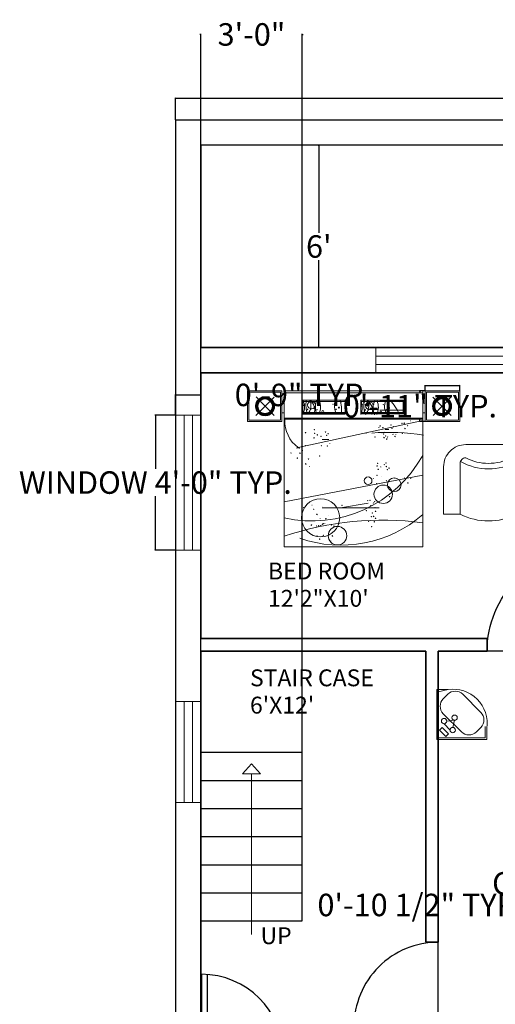
# Model space of a CAD drawing. Units: inches. Extents: x -11 to 443, y 65 to 743.
# Tile 7 of 10: x -11 to 158, y 392 to 743. Entities that reach past the tile are written whole.
import ezdxf

# ---------------------------------------------------------------- set-up
doc = ezdxf.new("R2010")
doc.units = ezdxf.units.IN
doc.header["$MEASUREMENT"] = 0
for name, color, linetype, lineweight in [('A-ANNO-DIMS', 2, 'Continuous', 18), ('A-ANNO-SYMB', 2, 'Continuous', 18), ('A-ANNO-TEXT', 2, 'Continuous', 18), ('A-AREA-IDEN', 2, 'Continuous', 18), ('A-DOOR', 4, 'Continuous', 25), ('A-FLOR-FIXT', 8, 'Continuous', 18), ('A-FLOR-STRS', 7, 'Continuous', 25), ('A-FURN-PATT', 8, 'Continuous', 9), ('A-GLAZ', 4, 'Continuous', 18), ('A-WALL', 7, 'Continuous', 35), ('A-WALL-SITE', 7, 'Continuous', 30), ('C-PROP', 3, 'Continuous', 30), ('Furniture', 7, 'Continuous', 15)]:
    doc.layers.add(name, color=color, linetype=linetype, lineweight=lineweight)
doc.styles.get("Standard").update_dxf_attribs({"font": 'italic8.shx'})
doc.dimstyles.get("Standard").update_dxf_attribs({"dimtxt": 8, "dimasz": 0.18, "dimexe": 0.18, "dimexo": 0.0625, "dimgap": 0.09, "dimtad": 0, "dimtih": 1, "dimtoh": 1, "dimzin": 0, "dimdsep": 46, "dimlunit": 3, "dimtxsty": 'Standard', "dimblk": 'CLOSEDBLANK', "dimcen": 0.09, "dimclrd": 6, "dimclre": 5, "dimclrt": 4, "dimadec": 0, "dimazin": 0, "dimtfac": 1, "dimtofl": 0, "dimtmove": 0, "dimatfit": 3, "dimfxl": 1, "dimtolj": 1, "dimtzin": 0, "dimarcsym": 0})

# ---------------------------------------------------------------- blocks, each defined once
blk = doc.blocks.new('_ClosedBlank')
at = {"color": 0, "linetype": 'ByBlock', "lineweight": -2}
for p, q in [((-1, 0.17), (0, 0)), ((-1, 0.17), (-1, -0.17)), ((0, 0), (-1, -0.17))]:
    blk.add_line(p, q, dxfattribs=at)
blk = doc.blocks.new('*D3')
at = {"layer": 'A-ANNO-DIMS', "color": 0, "lineweight": -2, "transparency": 16777216}
for p, q in [((95.1, 697.92), (94.99, 697.92)), ((95.17, 697.74), (95.17, 666.77)), ((95.17, 626.1), (95.17, 657.07)), ((95.1, 625.92), (94.99, 625.92))]:
    blk.add_line(p, q, dxfattribs=at)
at = {"layer": 'Defpoints', "color": 0, "lineweight": 100, "transparency": 16777216}
for p in [(95.17, 697.92), (95.17, 697.92), (95.17, 625.92)]:
    blk.add_point(p, dxfattribs=at)
at = {"layer": 'A-ANNO-DIMS', "color": 0, "lineweight": -2, "transparency": 16777216, "xscale": 0.18, "yscale": 0.18, "zscale": 0.18}
for p, rotation in [((95.17, 697.92), 90), ((95.17, 625.92), 270)]:
    blk.add_blockref('_ClosedBlank', p, dxfattribs=dict(at, rotation=rotation))
at = {"layer": 'A-ANNO-DIMS', "color": 0, "transparency": 16777216, "insert": (95.17, 661.92), "char_height": 8, "attachment_point": 5}
blk.add_mtext("\\A1;6'", dxfattribs=at)
blk = doc.blocks.new('*D5')
at = {"layer": 'A-ANNO-DIMS', "color": 0, "lineweight": -2, "transparency": 16777216}
for p, q in [((44.21, 706.98), (44.21, 714.84)), ((332.21, 706.98), (332.21, 714.84)), ((44.39, 714.66), (178.6, 714.66)), ((332.03, 714.66), (197.82, 714.66))]:
    blk.add_line(p, q, dxfattribs=at)
at = {"layer": 'Defpoints', "color": 0, "lineweight": 100, "transparency": 16777216}
for p in [(332.21, 714.66), (44.21, 706.92), (332.21, 706.92)]:
    blk.add_point(p, dxfattribs=at)
at = {"layer": 'A-ANNO-DIMS', "color": 0, "lineweight": -2, "transparency": 16777216, "xscale": 0.18, "yscale": 0.18, "zscale": 0.18, "rotation": 180}
blk.add_blockref('_ClosedBlank', (44.21, 714.66), dxfattribs=at)
at = {"layer": 'A-ANNO-DIMS', "color": 0, "lineweight": -2, "transparency": 16777216, "xscale": 0.18, "yscale": 0.18, "zscale": 0.18}
blk.add_blockref('_ClosedBlank', (332.21, 714.66), dxfattribs=at)
at = {"layer": 'A-ANNO-DIMS', "color": 0, "transparency": 16777216, "insert": (188.21, 714.66), "char_height": 8, "attachment_point": 5}
blk.add_mtext("\\A1;24'", dxfattribs=at)
blk = doc.blocks.new('DOOR-SWING-30')
for p, q in [((0, 30), (0, 0)), ((2, 29.93), (2, 0)), ((0, 0), (30, 0))]:
    blk.add_line(p, q)
blk.add_arc((0, 0), 30, 0, 90)
blk = doc.blocks.new('DOOR-SWING-36')
for p, q in [((36, 36), (0, 36)), ((0, 36), (0, 0)), ((35.94, 34), (0, 34))]:
    blk.add_line(p, q)
blk.add_arc((0, 36), 36, 270, 0)
blk = doc.blocks.new('WIN-48x9')
for p, q in [((0, 48), (0, 0)), ((9, 48), (0, 48)), ((3, 0), (3, 48)), ((6, 0), (6, 48)), ((9, 0), (9, 48)), ((0, 0), (9, 0))]:
    blk.add_line(p, q)
blk = doc.blocks.new('BED-DOUBLE')
for p, q in [((0.82, 54.51), (0, 54.51)), ((50.12, 55.53), (0.82, 55.53)), ((0.82, 55.53), (0.82, 0)), ((50.12, 54.78), (0.82, 54.78)), ((50.12, 0), (50.12, 55.53)), ((50.12, 0), (50.12, 55.53)), ((50.95, 54.51), (50.12, 54.51)), ((0.82, 51.08), (0, 51.08)), ((7.45, 52.2), (7.45, 47.27)), ((22.51, 52.2), (7.45, 52.2)), ((7.45, 51.71), (22.51, 51.71)), ((22.51, 47.27), (22.51, 52.2)), ((43.08, 52.21), (28.01, 52.21)), ((28.01, 52.21), (28.01, 47.28)), ((28.01, 51.71), (43.1, 51.71)), ((43.08, 52.14), (34.85, 52.14)), ((43.08, 47.28), (43.08, 52.21)), ((50.95, 51.08), (50.12, 51.08)), ((0.82, 47.66), (0, 47.66)), ((0.81, 45.69), (50.11, 45.69)), ((0.82, 45.79), (49.9, 45.79)), ((7.45, 47.77), (22.51, 47.77)), ((7.45, 47.56), (22.51, 47.56)), ((7.45, 47.35), (22.51, 47.35)), ((7.45, 47.27), (22.51, 47.27)), ((28.01, 47.77), (43.1, 47.77)), ((28.01, 47.56), (43.1, 47.56)), ((28.01, 47.35), (43.1, 47.35)), ((28.01, 47.28), (43.08, 47.28)), ((43.08, 48.66), (34.85, 48.66)), ((50.95, 47.66), (50.12, 47.66)), ((0.81, 45.48), (50.11, 45.48)), ((5.76, 35.31), (50.13, 44.94)), ((38, 41.71), (36.72, 41.71)), ((16.71, 38.23), (14.33, 38.23)), ((0.81, 16.07), (50.11, 25.52)), ((30.69, 15.53), (20.82, 13.88)), ((34.54, 13.88), (14.33, 13.88)), ((0.82, 0), (50.12, 0)), ((0.82, 0), (50.12, 0))]:
    blk.add_line(p, q)
for centre, radius in [((7.67, 50.33), 0.0548), ((7.99, 50.77), 0.0548), ((9.09, 50.77), 0.0548), ((10.51, 50.44), 1.37), ((10.62, 51.21), 0.0274), ((10.95, 51.64), 0.0274), ((12.05, 51.64), 0.0274), ((12.05, 50.88), 0.0274), ((18.18, 50.77), 0.0548), ((20.26, 49.56), 0.164), ((21.14, 51.64), 0.0274), ((28.25, 50.16), 0.0548), ((28.58, 50.6), 0.0548), ((29.68, 50.6), 0.0548), ((31.1, 50.27), 1.37), ((31.21, 51.03), 0.0274), ((31.53, 51.47), 0.0274), ((32.63, 51.47), 0.0274), ((32.63, 50.71), 0.0274), ((36.03, 50.6), 0.0548), ((38.11, 49.39), 0.164), ((41.72, 51.47), 0.0274), ((8.76, 48.47), 0.0822), ((9.09, 48.91), 0.0822), ((10.19, 48.91), 0.0822), ((12.48, 48.8), 0.0274), ((14.56, 48.14), 0.329), ((19.27, 48.91), 0.0822), ((29.35, 48.3), 0.0822), ((29.67, 48.74), 0.0822), ((30.77, 48.74), 0.0822), ((33.07, 48.63), 0.0274), ((35.15, 47.97), 0.329), ((37.12, 48.74), 0.0822), ((41.53, 45.6), 0.0822), ((34.49, 42.48), 0.0548), ((34.94, 42.97), 0.0822), ((35.9, 42.4), 0.0822), ((38.78, 43.35), 0.0822), ((39.16, 42.2), 0.0822), ((39.74, 42.78), 0.0822), ((42.72, 43.97), 0.0548), ((43.5, 44.01), 0.0822), ((43.81, 42.11), 0.0822), ((44.72, 43.1), 0.0274), ((45.68, 44.84), 0.0274), ((8.39, 40.62), 0.0822), ((11.37, 38.79), 0.0822), ((11.51, 41.72), 0.0548), ((11.65, 40.43), 0.0822), ((12.61, 39.86), 0.0822), ((13.92, 39.31), 0.0548), ((15.49, 40.82), 0.0822), ((15.87, 39.67), 0.0822), ((16.44, 40.24), 0.0822), ((29.94, 40.51), 0.0822), ((33.1, 39.09), 0.0822), ((35.59, 40.62), 0.0822), ((36.22, 40.19), 0.0548), ((36.35, 38.9), 0.0822), ((36.59, 41.14), 0.0274), ((36.93, 39.48), 0.0822), ((37.56, 39.06), 0.0548), ((39.48, 40), 0.0548), ((40.19, 39.28), 0.0822), ((40.52, 39.93), 0.0274), ((42.86, 40.37), 0.0822), ((5.33, 35.19), 0.0548), ((6.11, 35.23), 0.0822), ((8.29, 36.06), 0.0274), ((14.06, 35.98), 0.0548), ((16.11, 35.86), 0.0822), ((17.02, 36.86), 0.0274), ((37.31, 38.33), 0.0822), ((3.2, 33.44), 0.0548), ((5.48, 31.58), 0.0822), ((6.43, 33.33), 0.0822), ((7.34, 34.32), 0.0274), ((13.43, 32.33), 0.0548), ((8.49, 29.52), 0.0822), ((9.44, 31.26), 0.0822), ((9.72, 28.61), 0.0274), ((33.86, 28.77), 0.0822), ((34.05, 29.73), 0.0822), ((35.15, 28.44), 0.0274), ((36.41, 29.29), 0.0548), ((36.99, 29.87), 0.0548), ((37.12, 28.58), 0.0822), ((38.08, 28.01), 0.0822), ((30.66, 23.53), 1.37), ((33.81, 25.44), 0.0274), ((34.24, 27.62), 0.0822), ((35.53, 25.17), 0.0274), ((37.5, 27.43), 0.0822), ((39.97, 22.1), 2.46), ((43.71, 24.56), 0.0548), ((45.75, 24.45), 0.0822), ((32.57, 24.29), 0.0548), ((36.03, 18.71), 3.29), ((33.67, 22.43), 0.0822), ((37.18, 23.55), 0.0548), ((40.13, 24.42), 0.0274), ((44.8, 22.7), 0.0822), ((38.27, 17.83), 0.0822), ((13.75, 10.33), 6.79), ((10.67, 14.82), 0.0274), ((14.28, 14.25), 0.0274), ((21.36, 14.74), 0.0548), ((30.53, 16.48), 0.0548), ((31.31, 16.52), 0.0822), ((31.63, 14.62), 0.0822), ((32.54, 15.61), 0.0274), ((32.96, 16.06), 0.0548), ((7.71, 13.94), 0.0548), ((11.32, 13.38), 0.0548), ((12.42, 11.52), 0.0822), ((16.54, 11.02), 0.0274), ((30.03, 12.86), 0.0822), ((31.8, 10.77), 0.0548), ((32.19, 12.04), 0.0548), ((32.58, 10.82), 0.0822), ((33.15, 13.95), 0.0548), ((33.29, 12.66), 0.0822), ((10.5, 7.72), 0.0822), ((12.32, 7.47), 0.0548), ((13.09, 7.51), 0.0822), ((13.59, 10.14), 0.0548), ((13.76, 7.53), 0.0822), ((14.33, 8.01), 0.0822), ((14.68, 8.28), 0.0822), ((15.27, 8.25), 0.0274), ((15.63, 10.02), 0.0822), ((19.76, 3.97), 3.29), ((17.59, 7.82), 0.0822), ((18.55, 7.34), 0.0822), ((30.85, 9.03), 0.0548), ((31.95, 7.17), 0.0822), ((32.9, 8.91), 0.0822), ((33.29, 10.18), 0.0822), ((12.46, 3.87), 0.0822), ((14.32, 3.74), 0.0274), ((14.72, 4.1), 0.0822), ((17.98, 3.91), 0.0822), ((13.41, 2.75), 0.0822), ((17.39, 2.05), 0.0548)]:
    blk.add_circle(centre, radius)
for centre, radius, start, end in [((2.24, 49.73), 5.76, 334.6876, 25.3124), ((18.3, 50.59), 9.77, 171.2054, 199.8717), ((5.97, 50.26), 4.34, 316.473, 26.5351), ((7.41, 48.73), 4.24, 339.7755, 54.8367), ((18.16, 49.62), 6.28, 155.7867, 203.0598), ((7.63, 49.85), 6.08, 334.8533, 22.5945), ((24.13, 50.16), 5.46, 158.1924, 212.0094), ((10.49, 48.64), 10.74, 352.6491, 19.9229), ((22.83, 49.56), 5.76, 334.6876, 25.3124), ((38.89, 50.42), 9.77, 171.2054, 199.8717), ((26.55, 50.09), 4.34, 316.473, 26.5351), ((28, 48.56), 4.24, 339.7755, 54.8367), ((38.74, 49.45), 6.28, 155.7867, 203.0598), ((28.22, 49.68), 6.08, 334.8533, 22.5945), ((41.97, 49.99), 5.46, 158.1924, 212.0094), ((27.71, 41.52), 15.09, 21.7027, 44.6945), ((12.77, 44.72), 11.73, 177.3999, 233.2824), ((37.95, -36.79), 77.52, 80.7462, 94.4176), ((10.65, 54.27), 45.03, 257.3742, 331.1748), ((20.99, 44.94), 44.36, 250.6919, 311.0239), ((35.98, -101.04), 110.55, 82.6585, 108.5509)]:
    blk.add_arc(centre, radius, start, end)
blk = doc.blocks.new('NIGHTSTAND-LAMP')
for p, q in [((0, 10.9), (0, 0)), ((12.32, 10.9), (0, 10.9)), ((12.32, 0), (12.32, 10.9)), ((0.49, 10.41), (0.49, 0.49)), ((11.83, 10.41), (0.49, 10.41)), ((2.74, 8.7), (9.27, 2.17)), ((2.81, 2.1), (9.21, 8.77)), ((11.83, 0.49), (11.83, 10.41)), ((0.49, 0.49), (11.83, 0.49)), ((0, 0), (12.32, 0))]:
    blk.add_line(p, q)
for radius in [3.39, 2.6]:
    blk.add_circle((6.01, 5.43), radius)
blk = doc.blocks.new('LOVESEAT')
for p, q in [((0, 24.8, -27), (0, 7.87, -27)), ((0, 24.8, -27), (5.91, 24.8, -27)), ((5.91, 6.69, -27), (5.91, 24.8, -27)), ((25.98, 24.8, -27), (25.98, 6.69, -27)), ((25.98, 6.69, -27), (25.98, 24.8, -27)), ((46.06, 6.69, -27), (46.06, 24.8, -27)), ((46.06, 24.8, -27), (46.06, 6.69, -27)), ((46.06, 6.69, -27), (46.06, 24.8, -27)), ((51.97, 24.8, -27), (46.06, 24.8, -27)), ((51.97, 7.87, -27), (51.97, 24.8, -27)), ((7.87, 0, -27), (44.09, 0, -27))]:
    blk.add_line(p, q)
for centre, radius, start, end in [((15.94, 4.65, -27), 22.51, 63.519, 116.481), ((36.02, 4.65, -27), 22.51, 63.519, 116.481), ((7.87, 7.87, -27), 7.87, 180, 270), ((15.94, -10.84, -27), 19.5, 59.4911, 120.5089), ((36.02, -10.84, -27), 19.5, 59.4911, 120.5089), ((44.09, 7.87, -27), 7.87, 270, 0), ((7.87, 6.69, -27), 1.97, 180, 270), ((15.94, -10.84, -27), 17.53, 62.5861, 117.4139), ((24.02, 6.69, -27), 1.97, 270, 0), ((27.95, 6.69, -27), 1.97, 180, 270), ((36.02, -10.84, -27), 17.53, 62.5861, 117.4139), ((44.09, 6.69, -27), 1.97, 270, 0)]:
    blk.add_arc(centre, radius, start, end)
blk = doc.blocks.new('*D18')
at = {"layer": 'A-ANNO-DIMS', "color": 5, "lineweight": -2, "transparency": 16777216}
for p, q in [((44.15, 601.9), (36.83, 601.9)), ((44.15, 553.9), (36.83, 553.9))]:
    blk.add_line(p, q, dxfattribs=at)
at = {"layer": 'A-ANNO-DIMS', "color": 6, "lineweight": -2, "transparency": 16777216}
for p, q in [((37.01, 601.72), (37.01, 582.76)), ((37.01, 554.08), (37.01, 573.05))]:
    blk.add_line(p, q, dxfattribs=at)
at = {"layer": 'Defpoints', "color": 0, "lineweight": 100, "transparency": 16777216}
for p in [(37.01, 601.9), (44.21, 601.9), (44.21, 553.9)]:
    blk.add_point(p, dxfattribs=at)
at = {"layer": 'A-ANNO-DIMS', "color": 6, "lineweight": -2, "transparency": 16777216, "xscale": 0.18, "yscale": 0.18, "zscale": 0.18}
for p, rotation in [((37.01, 601.9), 90), ((37.01, 553.9), 270)]:
    blk.add_blockref('_ClosedBlank', p, dxfattribs=dict(at, rotation=rotation))
at = {"layer": 'A-ANNO-DIMS', "color": 4, "transparency": 16777216, "insert": (37.01, 577.9), "char_height": 8, "attachment_point": 5}
blk.add_mtext('\\A1;WINDOW 4\'-0" TYP.', dxfattribs=at)
blk = doc.blocks.new('*D19')
at = {"layer": 'A-ANNO-DIMS', "color": 5, "lineweight": -2, "transparency": 16777216}
for p, q in [((44.21, 601.97), (44.21, 609.28)), ((53.21, 601.97), (53.21, 609.28))]:
    blk.add_line(p, q, dxfattribs=at)
at = {"layer": 'A-ANNO-DIMS', "color": 6, "lineweight": -2, "transparency": 16777216}
for p, q in [((44.39, 609.1), (53.03, 609.1)), ((53.21, 609.1), (53.39, 609.1))]:
    blk.add_line(p, q, dxfattribs=at)
at = {"layer": 'Defpoints', "color": 0, "lineweight": 100, "transparency": 16777216}
for p in [(53.21, 609.1), (44.21, 601.9), (53.21, 601.9)]:
    blk.add_point(p, dxfattribs=at)
at = {"layer": 'A-ANNO-DIMS', "color": 6, "lineweight": -2, "transparency": 16777216, "xscale": 0.18, "yscale": 0.18, "zscale": 0.18, "rotation": 180}
blk.add_blockref('_ClosedBlank', (44.21, 609.1), dxfattribs=at)
at = {"layer": 'A-ANNO-DIMS', "color": 6, "lineweight": -2, "transparency": 16777216, "xscale": 0.18, "yscale": 0.18, "zscale": 0.18}
blk.add_blockref('_ClosedBlank', (53.21, 609.1), dxfattribs=at)
at = {"layer": 'A-ANNO-DIMS', "color": 4, "transparency": 16777216, "insert": (89.67, 609.1), "char_height": 8, "attachment_point": 5}
blk.add_mtext('\\A1;0\'-9" TYP.', dxfattribs=at)
blk = doc.blocks.new('*D26')
at = {"layer": 'A-ANNO-DIMS', "color": 5, "lineweight": -2, "transparency": 16777216}
for p, q in [((133.01, 610.6), (133.01, 612.57)), ((145.34, 610.6), (145.34, 612.57))]:
    blk.add_line(p, q, dxfattribs=at)
at = {"layer": 'A-ANNO-DIMS', "color": 6, "lineweight": -2, "transparency": 16777216}
for p, q in [((133.19, 612.39), (145.16, 612.39)), ((145.34, 612.39), (145.52, 612.39))]:
    blk.add_line(p, q, dxfattribs=at)
at = {"layer": 'Defpoints', "color": 0, "lineweight": 100, "transparency": 16777216}
for p in [(133.01, 610.54), (145.34, 612.39), (145.34, 610.54)]:
    blk.add_point(p, dxfattribs=at)
at = {"layer": 'A-ANNO-DIMS', "color": 6, "lineweight": -2, "transparency": 16777216, "xscale": 0.18, "yscale": 0.18, "zscale": 0.18, "rotation": 180}
blk.add_blockref('_ClosedBlank', (133.01, 612.39), dxfattribs=at)
at = {"layer": 'A-ANNO-DIMS', "color": 6, "lineweight": -2, "transparency": 16777216, "xscale": 0.18, "yscale": 0.18, "zscale": 0.18}
blk.add_blockref('_ClosedBlank', (145.34, 612.39), dxfattribs=at)
at = {"layer": 'A-ANNO-DIMS', "color": 4, "transparency": 16777216, "insert": (242.18, 612.39), "char_height": 8, "attachment_point": 5}
blk.add_mtext('\\A1;NIGHTSTAND 1\'-0 1/2" TYP.', dxfattribs=at)
blk = doc.blocks.new('*D27')
at = {"layer": 'A-ANNO-DIMS', "color": 5, "lineweight": -2, "transparency": 16777216}
for p, q in [((132.95, 610.54), (130.98, 610.54)), ((132.95, 599.64), (130.98, 599.64))]:
    blk.add_line(p, q, dxfattribs=at)
at = {"layer": 'A-ANNO-DIMS', "color": 6, "lineweight": -2, "transparency": 16777216}
for p, q in [((131.16, 610.36), (131.16, 609.94)), ((131.16, 599.82), (131.16, 600.24))]:
    blk.add_line(p, q, dxfattribs=at)
at = {"layer": 'Defpoints', "color": 0, "lineweight": 100, "transparency": 16777216}
for p in [(131.16, 610.54), (133.01, 610.54), (133.01, 599.64)]:
    blk.add_point(p, dxfattribs=at)
at = {"layer": 'A-ANNO-DIMS', "color": 6, "lineweight": -2, "transparency": 16777216, "xscale": 0.18, "yscale": 0.18, "zscale": 0.18}
for p, rotation in [((131.16, 610.54), 90), ((131.16, 599.64), 270)]:
    blk.add_blockref('_ClosedBlank', p, dxfattribs=dict(at, rotation=rotation))
at = {"layer": 'A-ANNO-DIMS', "color": 4, "transparency": 16777216, "insert": (131.16, 605.09), "char_height": 8, "attachment_point": 5}
blk.add_mtext('\\A1;0\'-11" TYP.', dxfattribs=at)
blk = doc.blocks.new('*D28')
at = {"layer": 'A-ANNO-DIMS', "color": 5, "lineweight": -2, "transparency": 16777216}
for p, q in [((196.6, 441.21), (198.5, 441.21)), ((196.6, 429.36), (198.5, 429.36))]:
    blk.add_line(p, q, dxfattribs=at)
at = {"layer": 'A-ANNO-DIMS', "color": 6, "lineweight": -2, "transparency": 16777216}
for p, q in [((198.32, 441.03), (198.32, 440.14)), ((198.32, 429.54), (198.32, 430.44))]:
    blk.add_line(p, q, dxfattribs=at)
at = {"layer": 'Defpoints', "color": 0, "lineweight": 100, "transparency": 16777216}
for p in [(196.54, 441.21), (196.54, 429.36), (198.32, 429.36)]:
    blk.add_point(p, dxfattribs=at)
at = {"layer": 'A-ANNO-DIMS', "color": 6, "lineweight": -2, "transparency": 16777216, "xscale": 0.18, "yscale": 0.18, "zscale": 0.18}
for p, rotation in [((198.32, 441.21), 90), ((198.32, 429.36), 270)]:
    blk.add_blockref('_ClosedBlank', p, dxfattribs=dict(at, rotation=rotation))
at = {"layer": 'A-ANNO-DIMS', "color": 4, "transparency": 16777216, "insert": (198.32, 435.29), "char_height": 8, "attachment_point": 5}
blk.add_mtext('\\A1;CHAIR 1\'-0" TYP.', dxfattribs=at)
blk = doc.blocks.new('*D29')
at = {"layer": 'A-ANNO-DIMS', "color": 6, "lineweight": -2, "transparency": 16777216}
for p, q in [((185.91, 427.58), (185.73, 427.58)), ((196.36, 427.58), (186.09, 427.58))]:
    blk.add_line(p, q, dxfattribs=at)
at = {"layer": 'A-ANNO-DIMS', "color": 5, "lineweight": -2, "transparency": 16777216}
for p, q in [((185.91, 429.3), (185.91, 427.4)), ((196.54, 429.3), (196.54, 427.4))]:
    blk.add_line(p, q, dxfattribs=at)
at = {"layer": 'Defpoints', "color": 0, "lineweight": 100, "transparency": 16777216}
for p in [(185.91, 429.36), (185.91, 427.58), (196.54, 429.36)]:
    blk.add_point(p, dxfattribs=at)
at = {"layer": 'A-ANNO-DIMS', "color": 6, "lineweight": -2, "transparency": 16777216, "xscale": 0.18, "yscale": 0.18, "zscale": 0.18, "rotation": 180}
blk.add_blockref('_ClosedBlank', (185.91, 427.58), dxfattribs=at)
at = {"layer": 'A-ANNO-DIMS', "color": 6, "lineweight": -2, "transparency": 16777216, "xscale": 0.18, "yscale": 0.18, "zscale": 0.18}
blk.add_blockref('_ClosedBlank', (196.54, 427.58), dxfattribs=at)
at = {"layer": 'A-ANNO-DIMS', "color": 4, "transparency": 16777216, "insert": (131.55, 427.58), "char_height": 8, "attachment_point": 5}
blk.add_mtext('\\A1;0\'-10 1/2" TYP.', dxfattribs=at)
blk = doc.blocks.new('*D40')
at = {"layer": 'A-ANNO-DIMS', "color": 6, "lineweight": -2, "transparency": 16777216}
for p, q in [((53.029187, 737.379289), (52.849187, 737.379289)), ((89.389187, 737.379289), (89.569187, 737.379289))]:
    blk.add_line(p, q, dxfattribs=at)
at = {"layer": 'A-ANNO-DIMS', "color": 5, "lineweight": -2, "transparency": 16777216}
for p, q in [((53.209187, 421.982289), (53.209187, 737.559289)), ((89.209187, 421.982289), (89.209187, 737.559289))]:
    blk.add_line(p, q, dxfattribs=at)
at = {"layer": 'Defpoints', "color": 0, "lineweight": 100, "transparency": 16777216}
for p in [(89.209187, 737.379289), (53.209187, 421.919789), (89.209187, 421.919789)]:
    blk.add_point(p, dxfattribs=at)
at = {"layer": 'A-ANNO-DIMS', "color": 6, "lineweight": -2, "transparency": 16777216, "xscale": 0.18, "yscale": 0.18, "zscale": 0.18}
blk.add_blockref('_ClosedBlank', (53.209187, 737.379289), dxfattribs=at)
at = {"layer": 'A-ANNO-DIMS', "color": 6, "lineweight": -2, "transparency": 16777216, "xscale": 0.18, "yscale": 0.18, "zscale": 0.18, "rotation": 180}
blk.add_blockref('_ClosedBlank', (89.209187, 737.379289), dxfattribs=at)
at = {"layer": 'A-ANNO-DIMS', "color": 4, "transparency": 16777216, "insert": (71.209187, 737.379289), "char_height": 8, "attachment_point": 5}
blk.add_mtext('\\A1;3\'-0"', dxfattribs=at)

msp = doc.modelspace()

# ---------------------------------------------------------------- hatches: boundary and pattern name
at = {"layer": 'A-FURN-PATT'}
h = msp.add_hatch(dxfattribs=at)
h.set_pattern_fill('ANSI37', color=256, scale=0.6260848, angle=45, style=0)
h.paths.add_polyline_path([(79.448, 605.07), (79.445, 605.203), (79.437, 605.335), (79.424, 605.468), (79.406, 605.6), (79.383, 605.731), (79.354, 605.861), (79.321, 605.989), (79.282, 606.117), (79.238, 606.242), (79.19, 606.366), (79.137, 606.488), (79.079, 606.608), (79.016, 606.725), (78.949, 606.84), (78.877, 606.952), (78.801, 607.061), (78.72, 607.167), (78.636, 607.27), (78.548, 607.369), (78.455, 607.465), (78.36, 607.558), (78.26, 607.646), (78.157, 607.73), (78.051, 607.811), (77.942, 607.887), (77.83, 607.959), (77.715, 608.026), (77.598, 608.088), (77.478, 608.147), (77.356, 608.2), (77.232, 608.248), (77.107, 608.292), (76.979, 608.331), (76.851, 608.364), (76.721, 608.393), (76.59, 608.416), (76.458, 608.434), (76.325, 608.447), (76.193, 608.455), (76.06, 608.458), (75.927, 608.455), (75.794, 608.447), (75.661, 608.434), (75.53, 608.416), (75.399, 608.393), (75.269, 608.364), (75.14, 608.331), (75.013, 608.292), (74.887, 608.248), (74.763, 608.2), (74.641, 608.147), (74.521, 608.088), (74.404, 608.026), (74.289, 607.959), (74.177, 607.887), (74.068, 607.811), (73.962, 607.73), (73.859, 607.646), (73.76, 607.558), (73.664, 607.465), (73.572, 607.369), (73.483, 607.27), (73.399, 607.167), (73.318, 607.061), (73.242, 606.952), (73.171, 606.84), (73.103, 606.725), (73.041, 606.608), (72.983, 606.488), (72.929, 606.366), (72.881, 606.242), (72.837, 606.117), (72.799, 605.989), (72.765, 605.861), (72.736, 605.731), (72.713, 605.6), (72.695, 605.468), (72.682, 605.335), (72.674, 605.203), (72.671, 605.07), (72.674, 604.937), (72.682, 604.804), (72.695, 604.671), (72.713, 604.539), (72.736, 604.409), (72.765, 604.279), (72.799, 604.15), (72.837, 604.022), (72.881, 603.897), (72.929, 603.773), (72.983, 603.651), (73.041, 603.531), (73.103, 603.414), (73.171, 603.299), (73.242, 603.187), (73.318, 603.078), (73.399, 602.972), (73.483, 602.869), (73.572, 602.77), (73.664, 602.674), (73.76, 602.581), (73.859, 602.493), (73.962, 602.409), (74.068, 602.328), (74.177, 602.252), (74.289, 602.181), (74.404, 602.113), (74.521, 602.051), (74.641, 601.992), (74.763, 601.939), (74.887, 601.891), (75.013, 601.847), (75.14, 601.808), (75.269, 601.775), (75.399, 601.746), (75.53, 601.723), (75.661, 601.705), (75.794, 601.692), (75.927, 601.684), (76.06, 601.681), (76.193, 601.684), (76.325, 601.692), (76.458, 601.705), (76.59, 601.723), (76.721, 601.746), (76.851, 601.775), (76.979, 601.808), (77.107, 601.847), (77.232, 601.891), (77.356, 601.939), (77.478, 601.992), (77.598, 602.051), (77.715, 602.113), (77.83, 602.181), (77.942, 602.252), (78.051, 602.328), (78.157, 602.409), (78.26, 602.493), (78.36, 602.581), (78.455, 602.674), (78.548, 602.77), (78.636, 602.869), (78.72, 602.972), (78.801, 603.078), (78.877, 603.187), (78.949, 603.299), (79.016, 603.414), (79.079, 603.531), (79.137, 603.651), (79.19, 603.773), (79.238, 603.897), (79.282, 604.022), (79.321, 604.15), (79.354, 604.279), (79.383, 604.409), (79.406, 604.539), (79.424, 604.671), (79.437, 604.804), (79.445, 604.937)])
h.paths.add_polyline_path([(78.664, 605.07), (78.662, 604.967), (78.656, 604.865), (78.646, 604.763), (78.632, 604.662), (78.614, 604.561), (78.592, 604.461), (78.567, 604.362), (78.537, 604.265), (78.503, 604.168), (78.466, 604.073), (78.425, 603.979), (78.38, 603.887), (78.332, 603.797), (78.281, 603.709), (78.225, 603.622), (78.167, 603.538), (78.105, 603.457), (78.04, 603.378), (77.972, 603.301), (77.901, 603.228), (77.828, 603.157), (77.751, 603.089), (77.672, 603.024), (77.591, 602.962), (77.507, 602.904), (77.421, 602.849), (77.332, 602.797), (77.242, 602.749), (77.15, 602.704), (77.056, 602.663), (76.961, 602.626), (76.865, 602.592), (76.767, 602.563), (76.668, 602.537), (76.568, 602.515), (76.467, 602.497), (76.366, 602.483), (76.264, 602.473), (76.162, 602.467), (76.06, 602.465), (75.957, 602.467), (75.855, 602.473), (75.753, 602.483), (75.652, 602.497), (75.551, 602.515), (75.452, 602.537), (75.353, 602.563), (75.255, 602.592), (75.158, 602.626), (75.063, 602.663), (74.969, 602.704), (74.877, 602.749), (74.787, 602.797), (74.699, 602.849), (74.612, 602.904), (74.529, 602.962), (74.447, 603.024), (74.368, 603.089), (74.291, 603.157), (74.218, 603.228), (74.147, 603.301), (74.079, 603.378), (74.014, 603.457), (73.952, 603.538), (73.894, 603.622), (73.839, 603.709), (73.787, 603.797), (73.739, 603.887), (73.694, 603.979), (73.653, 604.073), (73.616, 604.168), (73.582, 604.265), (73.553, 604.362), (73.527, 604.461), (73.505, 604.561), (73.487, 604.662), (73.473, 604.763), (73.463, 604.865), (73.457, 604.967), (73.455, 605.07), (73.457, 605.172), (73.463, 605.274), (73.473, 605.376), (73.487, 605.477), (73.505, 605.578), (73.527, 605.678), (73.553, 605.777), (73.582, 605.874), (73.616, 605.971), (73.653, 606.066), (73.694, 606.16), (73.739, 606.252), (73.787, 606.342), (73.839, 606.431), (73.894, 606.517), (73.952, 606.601), (74.014, 606.682), (74.079, 606.761), (74.147, 606.838), (74.218, 606.911), (74.291, 606.982), (74.368, 607.05), (74.447, 607.115), (74.529, 607.177), (74.612, 607.235), (74.699, 607.29), (74.787, 607.342), (74.877, 607.39), (74.969, 607.435), (75.063, 607.476), (75.158, 607.513), (75.255, 607.547), (75.353, 607.577), (75.452, 607.602), (75.551, 607.624), (75.652, 607.642), (75.753, 607.656), (75.855, 607.666), (75.957, 607.672), (76.06, 607.674), (76.162, 607.672), (76.264, 607.666), (76.366, 607.656), (76.467, 607.642), (76.568, 607.624), (76.668, 607.602), (76.767, 607.577), (76.865, 607.547), (76.961, 607.513), (77.056, 607.476), (77.15, 607.435), (77.242, 607.39), (77.332, 607.342), (77.421, 607.29), (77.507, 607.235), (77.591, 607.177), (77.672, 607.115), (77.751, 607.05), (77.828, 606.982), (77.901, 606.911), (77.972, 606.838), (78.04, 606.761), (78.105, 606.682), (78.167, 606.601), (78.225, 606.517), (78.281, 606.431), (78.332, 606.342), (78.38, 606.252), (78.425, 606.16), (78.466, 606.066), (78.503, 605.971), (78.537, 605.874), (78.567, 605.777), (78.592, 605.678), (78.614, 605.578), (78.632, 605.477), (78.646, 605.376), (78.656, 605.274), (78.662, 605.172)], flags=0)
h = msp.add_hatch(dxfattribs=at)
h.set_pattern_fill('ANSI37', color=256, scale=0.6260848, angle=45, style=0)
h.paths.add_polyline_path([(142.409, 605.07), (142.406, 605.203), (142.398, 605.335), (142.385, 605.468), (142.367, 605.6), (142.343, 605.731), (142.315, 605.861), (142.281, 605.989), (142.243, 606.117), (142.199, 606.242), (142.151, 606.366), (142.097, 606.488), (142.039, 606.608), (141.977, 606.725), (141.909, 606.84), (141.837, 606.952), (141.761, 607.061), (141.681, 607.167), (141.597, 607.27), (141.508, 607.369), (141.416, 607.465), (141.32, 607.558), (141.221, 607.646), (141.118, 607.73), (141.012, 607.811), (140.903, 607.887), (140.791, 607.959), (140.676, 608.026), (140.558, 608.088), (140.439, 608.147), (140.317, 608.2), (140.193, 608.248), (140.067, 608.292), (139.94, 608.331), (139.811, 608.364), (139.681, 608.393), (139.55, 608.416), (139.418, 608.434), (139.286, 608.447), (139.153, 608.455), (139.02, 608.458), (138.887, 608.455), (138.754, 608.447), (138.622, 608.434), (138.49, 608.416), (138.359, 608.393), (138.229, 608.364), (138.101, 608.331), (137.973, 608.292), (137.848, 608.248), (137.724, 608.2), (137.602, 608.147), (137.482, 608.088), (137.365, 608.026), (137.25, 607.959), (137.138, 607.887), (137.029, 607.811), (136.923, 607.73), (136.82, 607.646), (136.72, 607.558), (136.624, 607.465), (136.532, 607.369), (136.444, 607.27), (136.359, 607.167), (136.279, 607.061), (136.203, 606.952), (136.131, 606.84), (136.064, 606.725), (136.001, 606.608), (135.943, 606.488), (135.89, 606.366), (135.841, 606.242), (135.798, 606.117), (135.759, 605.989), (135.726, 605.861), (135.697, 605.731), (135.674, 605.6), (135.655, 605.468), (135.642, 605.335), (135.635, 605.203), (135.632, 605.07), (135.635, 604.937), (135.642, 604.804), (135.655, 604.671), (135.674, 604.539), (135.697, 604.409), (135.726, 604.279), (135.759, 604.15), (135.798, 604.022), (135.841, 603.897), (135.89, 603.773), (135.943, 603.651), (136.001, 603.531), (136.064, 603.414), (136.131, 603.299), (136.203, 603.187), (136.279, 603.078), (136.359, 602.972), (136.444, 602.869), (136.532, 602.77), (136.624, 602.674), (136.72, 602.581), (136.82, 602.493), (136.923, 602.409), (137.029, 602.328), (137.138, 602.252), (137.25, 602.181), (137.365, 602.113), (137.482, 602.051), (137.602, 601.992), (137.724, 601.939), (137.848, 601.891), (137.973, 601.847), (138.101, 601.808), (138.229, 601.775), (138.359, 601.746), (138.49, 601.723), (138.622, 601.705), (138.754, 601.692), (138.887, 601.684), (139.02, 601.681), (139.153, 601.684), (139.286, 601.692), (139.418, 601.705), (139.55, 601.723), (139.681, 601.746), (139.811, 601.775), (139.94, 601.808), (140.067, 601.847), (140.193, 601.891), (140.317, 601.939), (140.439, 601.992), (140.558, 602.051), (140.676, 602.113), (140.791, 602.181), (140.903, 602.252), (141.012, 602.328), (141.118, 602.409), (141.221, 602.493), (141.32, 602.581), (141.416, 602.674), (141.508, 602.77), (141.597, 602.869), (141.681, 602.972), (141.761, 603.078), (141.837, 603.187), (141.909, 603.299), (141.977, 603.414), (142.039, 603.531), (142.097, 603.651), (142.151, 603.773), (142.199, 603.897), (142.243, 604.022), (142.281, 604.15), (142.315, 604.279), (142.343, 604.409), (142.367, 604.539), (142.385, 604.671), (142.398, 604.804), (142.406, 604.937)])
h.paths.add_polyline_path([(141.625, 605.07), (141.623, 604.967), (141.617, 604.865), (141.607, 604.763), (141.593, 604.662), (141.575, 604.561), (141.553, 604.461), (141.527, 604.362), (141.498, 604.265), (141.464, 604.168), (141.427, 604.073), (141.386, 603.979), (141.341, 603.887), (141.293, 603.797), (141.241, 603.709), (141.186, 603.622), (141.128, 603.538), (141.066, 603.457), (141.001, 603.378), (140.933, 603.301), (140.862, 603.228), (140.788, 603.157), (140.712, 603.089), (140.633, 603.024), (140.551, 602.962), (140.467, 602.904), (140.381, 602.849), (140.293, 602.797), (140.203, 602.749), (140.111, 602.704), (140.017, 602.663), (139.922, 602.626), (139.825, 602.592), (139.727, 602.563), (139.628, 602.537), (139.528, 602.515), (139.428, 602.497), (139.326, 602.483), (139.225, 602.473), (139.123, 602.467), (139.02, 602.465), (138.918, 602.467), (138.816, 602.473), (138.714, 602.483), (138.613, 602.497), (138.512, 602.515), (138.412, 602.537), (138.313, 602.563), (138.215, 602.592), (138.119, 602.626), (138.023, 602.663), (137.93, 602.704), (137.838, 602.749), (137.747, 602.797), (137.659, 602.849), (137.573, 602.904), (137.489, 602.962), (137.408, 603.024), (137.329, 603.089), (137.252, 603.157), (137.178, 603.228), (137.107, 603.301), (137.04, 603.378), (136.975, 603.457), (136.913, 603.538), (136.854, 603.622), (136.799, 603.709), (136.748, 603.797), (136.699, 603.887), (136.655, 603.979), (136.614, 604.073), (136.576, 604.168), (136.543, 604.265), (136.513, 604.362), (136.487, 604.461), (136.465, 604.561), (136.448, 604.662), (136.433, 604.763), (136.423, 604.865), (136.417, 604.967), (136.415, 605.07), (136.417, 605.172), (136.423, 605.274), (136.433, 605.376), (136.448, 605.477), (136.465, 605.578), (136.487, 605.678), (136.513, 605.777), (136.543, 605.874), (136.576, 605.971), (136.614, 606.066), (136.655, 606.16), (136.699, 606.252), (136.748, 606.342), (136.799, 606.431), (136.854, 606.517), (136.913, 606.601), (136.975, 606.682), (137.04, 606.761), (137.107, 606.838), (137.178, 606.911), (137.252, 606.982), (137.329, 607.05), (137.408, 607.115), (137.489, 607.177), (137.573, 607.235), (137.659, 607.29), (137.747, 607.342), (137.838, 607.39), (137.93, 607.435), (138.023, 607.476), (138.119, 607.513), (138.215, 607.547), (138.313, 607.577), (138.412, 607.602), (138.512, 607.624), (138.613, 607.642), (138.714, 607.656), (138.816, 607.666), (138.918, 607.672), (139.02, 607.674), (139.123, 607.672), (139.225, 607.666), (139.326, 607.656), (139.428, 607.642), (139.528, 607.624), (139.628, 607.602), (139.727, 607.577), (139.825, 607.547), (139.922, 607.513), (140.017, 607.476), (140.111, 607.435), (140.203, 607.39), (140.293, 607.342), (140.381, 607.29), (140.467, 607.235), (140.551, 607.177), (140.633, 607.115), (140.712, 607.05), (140.788, 606.982), (140.862, 606.911), (140.933, 606.838), (141.001, 606.761), (141.066, 606.682), (141.128, 606.601), (141.186, 606.517), (141.241, 606.431), (141.293, 606.342), (141.341, 606.252), (141.386, 606.16), (141.427, 606.066), (141.464, 605.971), (141.498, 605.874), (141.527, 605.777), (141.553, 605.678), (141.575, 605.578), (141.593, 605.477), (141.607, 605.376), (141.617, 605.274), (141.623, 605.172)], flags=0)

# ---------------------------------------------------------------- linework, layer by layer
at = {"layer": 'A-ANNO-SYMB'}
for p, q in [((67.967, 474.261), (71.209, 477.775)), ((74.452, 474.261), (71.209, 477.775)), ((71.209, 474.261), (67.967, 474.261)), ((71.209, 417.056), (71.209, 474.261)), ((71.209, 474.261), (74.452, 474.261))]:
    msp.add_line(p, q, dxfattribs=at)
at = {"layer": 'A-DOOR'}
for p, q in [((53.43, 402.92), (53.43, 373.92)), ((55.43, 402.851), (55.43, 373.92))]:
    msp.add_line(p, q, dxfattribs=at)
msp.add_arc((53.43, 373.92), 29, 0, 90, dxfattribs=at)
at = {"layer": 'A-FLOR-FIXT'}
for p, q in [((137.236, 504.228), (137.236, 486.511)), ((141.173, 504.228), (137.236, 504.228)), ((137.662, 503.379), (141.173, 504.228)), ((137.662, 487.066), (137.662, 503.379)), ((139.469, 500.97), (141.07, 502.571)), ((146.415, 502.571), (152.854, 496.132)), ((145.908, 489.186), (139.469, 495.625)), ((138.108, 489.818), (139.042, 490.752)), ((139.042, 490.752), (141.302, 488.491)), ((141.893, 489.822), (139.752, 492.078)), ((140.693, 493.018), (143.493, 493.29)), ((142.833, 490.762), (143.493, 493.29)), ((152.854, 490.787), (151.253, 489.186)), ((154.386, 487.066), (154.386, 491.145)), ((137.662, 487.066), (154.386, 487.066)), ((140.368, 487.558), (138.108, 489.818)), ((141.302, 488.491), (140.368, 487.558)), ((154.952, 486.511), (154.952, 490.448)), ((137.236, 486.511), (154.952, 486.511))]:
    msp.add_line(p, q, dxfattribs=at)
for centre in [(143.493, 494.231), (139.752, 493.018), (142.833, 489.822)]:
    msp.add_circle(centre, 0.94, dxfattribs=at)
for centre, radius, start, end in [((143.743, 499.899), 3.78, 45, 135), ((142.963, 492.238), 12.123, 351.50989, 98.49011), ((142.141, 498.298), 3.78, 135, 225), ((150.182, 493.46), 3.78, 315, 45), ((148.58, 491.859), 3.78, 225, 315)]:
    msp.add_arc(centre, radius, start, end, dxfattribs=at)
at = {"layer": 'A-FLOR-STRS'}
for p, q in [((53.209, 517.92), (53.209, 481.92)), ((53.209, 481.92), (89.209, 481.92)), ((89.209, 421.92), (89.209, 481.92)), ((53.209, 471.92), (89.209, 471.92)), ((53.209, 461.92), (89.209, 461.92)), ((53.209, 451.92), (89.209, 451.92)), ((53.209, 441.92), (89.209, 441.92)), ((53.209, 431.92), (89.209, 431.92)), ((53.209, 421.92), (89.209, 421.92))]:
    msp.add_line(p, q, dxfattribs=at)
at = {"layer": 'A-GLAZ'}
for p, q in [((44.209, 500.009), (44.209, 464.009)), ((53.209, 500.009), (44.209, 500.009)), ((44.209, 500.009), (48.709, 500.009)), ((47.209, 500.009), (47.209, 464.009)), ((50.209, 500.009), (50.209, 464.009)), ((53.209, 464.009), (53.209, 500.009)), ((44.209, 464.009), (53.209, 464.009))]:
    msp.add_line(p, q, dxfattribs=at)
at = {"layer": 'A-WALL'}
for p, q in [((323.209, 625.92), (53.209, 625.92)), ((53.209, 616.92), (53.209, 522.42)), ((53.209, 616.92), (53.209, 522.42)), ((194.709, 616.92), (53.209, 616.92)), ((53.209, 522.42), (155.085, 522.42)), ((155.085, 522.42), (155.085, 517.92)), ((53.209, 517.92), (133.209, 517.92)), ((53.209, 517.92), (53.209, 378.42)), ((133.209, 517.92), (133.209, 414.35)), ((137.709, 517.92), (137.709, 414.35)), ((137.709, 517.92), (155.085, 517.92)), ((137.709, 414.35), (133.209, 414.35))]:
    msp.add_line(p, q, dxfattribs=at)
at = {"layer": 'A-WALL-SITE'}
for p, q in [((323.209, 697.92), (53.209, 697.92)), ((53.209, 697.92), (53.209, 625.92))]:
    msp.add_line(p, q, dxfattribs=at)
at = {"layer": 'C-PROP'}
msp.add_lwpolyline([(44.209, 106.92), (332.209, 106.92), (332.209, 706.92), (44.209, 706.92)], close=True, dxfattribs=at)

# ---------------------------------------------------------------- block references
at = {"layer": 'A-DOOR', "extrusion": (0, 0, -1), "zscale": -1, "rotation": 90.00000000000014}
msp.add_blockref('DOOR-SWING-36', (-155.086, 517.92), dxfattribs=at)
at = {"layer": 'A-DOOR', "rotation": 89.99999999999991}
msp.add_blockref('DOOR-SWING-30', (137.709, 384.35), dxfattribs=at)
at = {"layer": 'A-GLAZ', "rotation": 90.00000000000003}
msp.add_blockref('WIN-48x9', (163.513, 616.92), dxfattribs=at)
at = {"layer": 'A-GLAZ'}
msp.add_blockref('WIN-48x9', (44.209, 553.904), dxfattribs=at)
at = {"layer": 'Furniture', "extrusion": (0, 0, -1), "zscale": -1}
msp.add_blockref('NIGHTSTAND-LAMP', (-82.067, 599.636), dxfattribs=at)
at = {"layer": 'Furniture'}
for name, p in [('BED-DOUBLE', (82.067, 555.029)), ('NIGHTSTAND-LAMP', (133.013, 599.636))]:
    msp.add_blockref(name, p, dxfattribs=at)
at = {"layer": 'Furniture', "rotation": 180}
msp.add_blockref('LOVESEAT', (191.555, 591.409), dxfattribs=at)

# ---------------------------------------------------------------- texts
at = {"layer": 'A-ANNO-TEXT'}
msp.add_text('UP', height=6, dxfattribs=at).set_placement((74.432, 413.635))
at = {"layer": 'A-AREA-IDEN'}
for s, p in [('BED ROOM', (77.091, 543.418)), ('12\'2"X10\'', (77.091, 533.704)), ('STAIR CASE', (70.682, 505.413)), ("6'X12'", (70.682, 495.699))]:
    msp.add_text(s, height=6, dxfattribs=at).set_placement(p)

# ---------------------------------------------------------------- dimensions: what is measured, and where the dimension line sits
at = {"layer": 'A-ANNO-DIMS'}
for base, p1, p2, override, picture, middle in [((89.209, 737.379), (53.209, 421.92), (89.209, 421.92), {"dimdec": 1, "dimlfac": 1, "dimrnd": 0, "dimzin": 1, "dimdsep": 46, "dimlunit": 4, "dimfrac": 2}, '*D40', (71.209, 737.379)), ((332.209, 714.661), (44.209, 706.92), (332.209, 706.92), {"dimclrd": 0, "dimclre": 0, "dimclrt": 0}, '*D5', (188.209, 714.661))]:
    dim = msp.add_linear_dim(base=base, p1=p1, p2=p2, dimstyle='Standard', override=override, dxfattribs=at)
    dim.commit()
    dim.dimension.update_dxf_attribs({"geometry": picture, "text_midpoint": middle})
dim = msp.add_linear_dim(base=(95.165, 697.92), p1=(95.165, 625.92), p2=(95.165, 697.92), angle=90, dimstyle='Standard', override={"dimclrd": 0, "dimclre": 0, "dimclrt": 0}, dxfattribs=at)
dim.commit()
dim.dimension.update_dxf_attribs({"geometry": '*D3', "text_midpoint": (95.165, 661.92)})
for base, p1, p2, text, picture, middle in [((145.337, 612.387), (133.013, 610.539), (145.337, 610.539), 'NIGHTSTAND <> TYP.', '*D26', (242.179, 612.387)), ((53.209, 609.104), (44.209, 601.904), (53.209, 601.904), '<> TYP.', '*D19', (89.67, 609.104))]:
    dim = msp.add_linear_dim(base=base, p1=p1, p2=p2, text=text, dimstyle='Standard', override={"dimdec": 1, "dimlfac": 1, "dimrnd": 0, "dimzin": 1, "dimdsep": 46, "dimlunit": 4, "dimfrac": 2}, dxfattribs=at)
    dim.commit()
    dim.dimension.update_dxf_attribs({"geometry": picture, "text_midpoint": middle})
for base, p1, p2, angle, text, picture, middle in [((131.164, 610.539), (133.013, 599.636), (133.013, 610.539), 90, '<> TYP.', '*D27', (131.164, 605.087)), ((37.009, 601.904), (44.209, 553.904), (44.209, 601.904), 90, 'WINDOW <> TYP.', '*D18', (37.009, 577.904)), ((198.318, 429.362), (196.54, 441.214), (196.54, 429.362), 270, 'CHAIR <> TYP.', '*D28', (198.318, 435.288)), ((185.911, 427.584), (196.54, 429.362), (185.911, 429.362), 180, '<> TYP.', '*D29', (131.545, 427.584))]:
    dim = msp.add_linear_dim(base=base, p1=p1, p2=p2, angle=angle, text=text, dimstyle='Standard', override={"dimdec": 1, "dimlfac": 1, "dimrnd": 0, "dimzin": 1, "dimdsep": 46, "dimlunit": 4, "dimfrac": 2}, dxfattribs=at)
    dim.commit()
    dim.dimension.update_dxf_attribs({"geometry": picture, "text_midpoint": middle})

doc.saveas('drawing.dxf')
